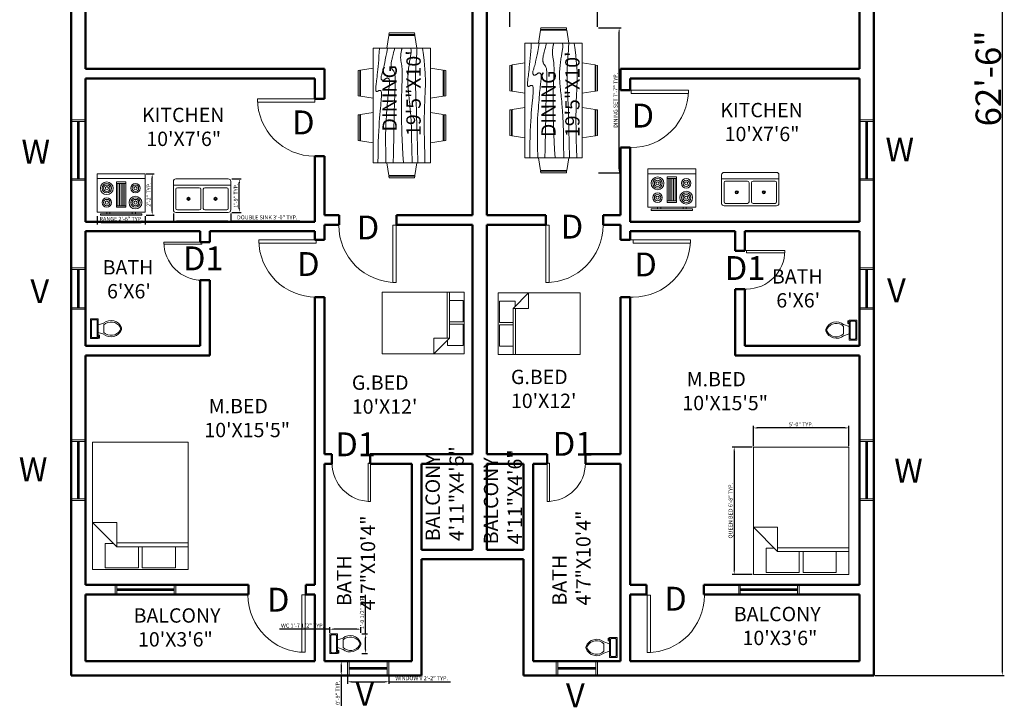
# Model space of a CAD drawing. Units: inches. Extents: x -7040 to -4088, y 6092 to 7645.
# Tile 10 of 11: x -4706 to -4088, y 6744 to 7176. Entities that reach past the tile are written whole.
import ezdxf

# ---------------------------------------------------------------- set-up
doc = ezdxf.new("R2010")
doc.units = ezdxf.units.IN
for name, color, linetype, lineweight in [('A-ANNO-DIMS', 2, 'Continuous', 18), ('A-ANNO-TEXT', 7, 'Continuous', 25), ('A-AREA-IDEN', 3, 'Continuous', 25), ('A-DOOR', 3, 'Continuous', 18), ('A-FLOR-FIXT', 9, 'Continuous', 13), ('A-FURN', 8, 'Continuous', 13), ('A-GLAZ', 4, 'Continuous', 18), ('A-WALL', 7, 'Continuous', 50)]:
    doc.layers.add(name, color=color, linetype=linetype, lineweight=lineweight)
doc.styles.get("Standard").update_dxf_attribs({"font": 'arial.ttf'})
doc.dimstyles.new('ISO-25', dxfattribs={"dimtxt": 2.5, "dimasz": 2.5, "dimexe": 1.25, "dimexo": 0.625, "dimtad": 1, "dimdec": 0, "dimlunit": 3, "dimtxsty": 'Standard', "dimcen": 2.5, "dimadec": 0, "dimazin": 0, "dimtfac": 1, "dimtdec": 0, "dimtmove": 0, "dimatfit": 3, "dimfxl": 1, "dimarcsym": 0})

# ---------------------------------------------------------------- blocks, each defined once
blk = doc.blocks.new('*U8')
for p, q in [((0, 0), (0, -100)), ((750, 0), (750, -100))]:
    blk.add_line(p, q)
blk.add_lwpolyline([(0, 0), (0, 750), (43.75, 750), (43.75, 0)], close=True)
blk.add_arc((0, 0), 750, 0, 90)
blk = doc.blocks.new('Bed - Queen')
for p, q in [((0, -80.00003), (0, 0)), ((0, 0), (59.99999, 0)), ((59.99999, 0), (59.99999, -80.00003)), ((7.99999, -1.2), (28.79998, -1.2)), ((7.99999, -14.4), (7.99999, -1.2)), ((28.79998, -1.2), (28.79998, -14.4)), ((31.19999, -1.2), (51.99999, -1.2)), ((31.19999, -14.4), (31.19999, -1.2)), ((51.99999, -1.2), (51.99999, -16.4)), ((0, -14.4), (44.8, -14.4)), ((44.8, -16.8), (0, -16.8)), ((59.99999, -29.6), (44.8, -14.4)), ((44.8, -14.4), (44.8, -29.6)), ((51.99999, -16.4), (46.79936, -16.4)), ((44.8, -29.6), (59.99999, -29.6)), ((59.99999, -80.00003), (0, -80.00003))]:
    blk.add_line(p, q)
blk = doc.blocks.new('Dining Set - 36 x 72 in.')
for p, q in [((-22.2343, 26.00059), (-23.4847, 17.99762)), ((-22.2304, 26), (-5.7608, 26)), ((-22, 27.5), (-22.1562, 26.50042)), ((-5.8416, 26.5), (-22.1534, 26.5)), ((-22, 27.5), (-6, 27.5)), ((-5.8437, 26.49966), (-6, 27.5)), ((-4.5152, 17.99762), (-5.7655, 25.99926)), ((5.7657, 26.00059), (4.5153, 17.99762)), ((5.7696, 26), (22.2392, 26)), ((6, 27.5), (5.8438, 26.50042)), ((22.1584, 26.5), (5.8466, 26.5)), ((6, 27.5), (22, 27.5)), ((22.1563, 26.49966), (22, 27.5)), ((23.4848, 17.99762), (22.2345, 25.99926)), ((36, 18), (-36, 18)), ((-36, 18), (-36, -18)), ((36, -18), (36, 18)), ((-45.5, 8), (-44.5004, 8.15617)), ((-45.5, 8), (-45.5, -8)), ((-44.5, -8.15843), (-44.5, 8.15338)), ((-44.0006, 8.23428), (-35.9976, 9.48474)), ((-44, 8.23041), (-44, -8.23915)), ((44.0006, 8.23428), (35.9976, 9.48474)), ((44, 8.23041), (44, -8.23915)), ((44.5, -8.15843), (44.5, 8.15338)), ((45.5, 8), (44.5005, 8.15617)), ((45.5, 8), (45.5, -8)), ((-44.4997, -8.15631), (-45.5, -8)), ((-35.9976, -9.48476), (-43.9993, -8.2345)), ((35.9976, -9.48476), (43.9993, -8.2345)), ((44.4997, -8.15631), (45.5, -8)), ((-36, -18), (36, -18)), ((-22.2343, -26.0006), (-23.4847, -17.99762)), ((-4.5152, -17.99762), (-5.7655, -25.99928)), ((5.7657, -26.0006), (4.5153, -17.99762)), ((23.4848, -17.99762), (22.2345, -25.99928)), ((-22.2304, -26), (-5.7608, -26)), ((-22, -27.5), (-22.1562, -26.50044)), ((-5.8416, -26.5), (-22.1534, -26.5)), ((-22, -27.5), (-6, -27.5)), ((-5.8437, -26.49967), (-6, -27.5)), ((5.7696, -26), (22.2392, -26)), ((6, -27.5), (5.8438, -26.50044)), ((22.1584, -26.5), (5.8466, -26.5)), ((6, -27.5), (22, -27.5)), ((22.1563, -26.49967), (22, -27.5))]:
    blk.add_line(p, q)
for points in [[(-36, 15), (-31.1772, 14.97754), (-26.8079, 14.91406), (-22.8538, 14.81543), (-19.276, 14.6875), (-16.0362, 14.53613), (-13.0957, 14.36718), (-10.4159, 14.18652), (-7.9583, 14), (-5.6904, 13.81315), (-3.6035, 13.63021), (-1.6954, 13.45508), (0.0365, 13.29166), (1.5945, 13.14388), (2.9811, 13.01562), (4.1988, 12.9108), (5.25, 12.83333), (6.1393, 12.78613), (6.8802, 12.76823), (7.4883, 12.77767), (7.9792, 12.8125), (8.3685, 12.87077), (8.6719, 12.95052), (8.9049, 13.0498), (9.0833, 13.16666), (9.2205, 13.29899), (9.3216, 13.44401), (9.3895, 13.59879), (9.4271, 13.76041), (9.4373, 13.92594), (9.4232, 14.09245), (9.3875, 14.257), (9.3333, 14.41666), (9.2638, 14.56917), (9.1836, 14.71484), (9.0975, 14.85465), (9.0104, 14.98958), (8.9272, 15.1206), (8.8529, 15.2487), (8.7922, 15.37483), (8.75, 15.5), (8.7305, 15.62467), (8.7344, 15.74739), (8.7617, 15.86621), (8.8125, 15.97916), (8.8867, 16.08431), (8.9844, 16.17968), (9.1055, 16.26334), (9.25, 16.33333), (9.4189, 16.38802), (9.6172, 16.42708), (9.8506, 16.45052), (10.125, 16.45833), (10.4463, 16.45052), (10.8203, 16.42708), (11.2529, 16.38802), (11.75, 16.33333), (12.3184, 16.26318), (12.9694, 16.17838), (13.7151, 16.07991), (14.5677, 15.96875), (15.5395, 15.84586), (16.6426, 15.71224), (17.8893, 15.56884), (19.2917, 15.41666), (20.859, 15.25667), (22.5879, 15.08984), (24.4721, 14.91715), (26.5052, 14.73958), (28.6809, 14.5581), (30.9929, 14.3737), (33.4347, 14.18733), (36, 14)], [(-36, 10), (-28.9766, 10.14274), (-23.1725, 10.20442), (-18.4241, 10.19775), (-14.5677, 10.13541), (-11.4399, 10.03011), (-8.877, 9.89453), (-6.7154, 9.74137), (-4.7917, 9.58333), (-2.9698, 9.43082), (-1.2246, 9.28515), (0.4415, 9.14534), (2.026, 9.01041), (3.5266, 8.87939), (4.9408, 8.7513), (6.266, 8.62516), (7.5, 8.5), (8.6411, 8.37549), (9.6914, 8.2539), (10.6538, 8.13818), (11.5312, 8.03125), (12.3267, 7.93603), (13.043, 7.85547), (13.6831, 7.79248), (14.25, 7.75), (14.7471, 7.7303), (15.1797, 7.73307), (15.5537, 7.75732), (15.875, 7.80208), (16.1494, 7.86637), (16.3828, 7.94922), (16.5811, 8.04964), (16.75, 8.16666), (16.8944, 8.29915), (17.0143, 8.44531), (17.1089, 8.60319), (17.1771, 8.77083), (17.218, 8.94629), (17.2305, 9.1276), (17.2137, 9.31282), (17.1667, 9.5), (17.0895, 9.6875), (16.987, 9.875), (16.8649, 10.0625), (16.7292, 10.25), (16.5856, 10.4375), (16.4401, 10.625), (16.2985, 10.8125), (16.1667, 11), (16.05, 11.18733), (15.9518, 11.3737), (15.8752, 11.5581), (15.8229, 11.73958), (15.798, 11.91715), (15.8034, 12.08984), (15.842, 12.25667), (15.9167, 12.41666), (16.0295, 12.56836), (16.1784, 12.70833), (16.3605, 12.83268), (16.5729, 12.9375), (16.8127, 13.01888), (17.0768, 13.07291), (17.3625, 13.0957), (17.6667, 13.08333), (17.9894, 13.03312), (18.3418, 12.94726), (18.7382, 12.82918), (19.1927, 12.68229), (19.7195, 12.51001), (20.3327, 12.31575), (21.0465, 12.10294), (21.875, 11.875), (22.8357, 11.63354), (23.959, 11.37304), (25.2786, 11.08618), (26.8282, 10.76562), (28.6414, 10.40405), (30.752, 9.99414), (33.1936, 9.52856), (36, 9)], [(-36, 5.5), (-30.7157, 5.3348), (-26.069, 5.20963), (-21.9946, 5.11767), (-18.4271, 5.05208), (-15.3009, 5.00602), (-12.5508, 4.97265), (-10.1112, 4.94515), (-7.9167, 4.91666), (-5.909, 4.88167), (-4.0586, 4.83984), (-2.3429, 4.79215), (-0.7396, 4.73958), (0.7739, 4.6831), (2.22, 4.6237), (3.6213, 4.56233), (5, 4.5), (6.373, 4.43782), (7.7344, 4.3776), (9.0723, 4.32129), (10.375, 4.27083), (11.6309, 4.22819), (12.8281, 4.19531), (13.9551, 4.17415), (15, 4.16666), (15.954, 4.17448), (16.819, 4.19791), (17.6001, 4.23698), (18.3021, 4.29166), (18.9299, 4.36198), (19.4883, 4.44791), (19.9823, 4.54948), (20.4167, 4.66666), (20.7969, 4.79899), (21.1302, 4.94401), (21.4245, 5.09879), (21.6875, 5.26041), (21.9271, 5.42594), (22.1511, 5.59245), (22.3672, 5.757), (22.5834, 5.91666), (22.8065, 6.06868), (23.0404, 6.21093), (23.2879, 6.34147), (23.5521, 6.45833), (23.8358, 6.55957), (24.142, 6.64323), (24.4735, 6.70735), (24.8334, 6.75), (25.2235, 6.76969), (25.642, 6.76692), (26.0858, 6.74267), (26.5521, 6.69791), (27.0379, 6.63362), (27.5404, 6.55078), (28.0565, 6.45036), (28.5834, 6.33333), (29.1242, 6.19987), (29.7071, 6.04687), (30.3661, 5.87044), (31.1354, 5.66666), (32.0493, 5.43164), (33.142, 5.16146), (34.4475, 4.85221), (36, 4.5)], [(-36, -1), (-30.7915, -0.6591), (-26.0195, -0.38216), (-21.6519, -0.16284), (-17.6563, 0.00521), (-14.0005, 0.12833), (-10.6523, 0.21289), (-7.5796, 0.26522), (-4.75, 0.29166), (-2.134, 0.29793), (0.2878, 0.28711), (2.5317, 0.26163), (4.6146, 0.22396), (6.5529, 0.17651), (8.3633, 0.12174), (10.0623, 0.06209), (11.6667, 0), (13.1899, -0.06201), (14.6341, -0.1211), (15.9982, -0.17432), (17.2813, -0.21875), (18.4823, -0.25147), (19.6003, -0.26953), (20.6343, -0.27002), (21.5834, -0.25), (22.4481, -0.20768), (23.2357, -0.14584), (23.9549, -0.06836), (24.6146, 0.02083), (25.2235, 0.11784), (25.7904, 0.21875), (26.3241, 0.31966), (26.8334, 0.41666), (27.3265, 0.50618), (27.8099, 0.58593), (28.2894, 0.65397), (28.7709, 0.70833), (29.2601, 0.74707), (29.763, 0.76823), (30.2855, 0.76985), (30.8334, 0.75), (31.4088, 0.70784), (31.9994, 0.64713), (32.589, 0.57275), (33.1615, 0.48958), (33.7008, 0.4025), (34.1908, 0.3164), (34.6153, 0.23616), (34.9584, 0.16666), (35.2099, 0.11165), (35.3848, 0.07031), (35.504, 0.04069), (35.5886, 0.02083), (35.6594, 0.00879), (35.7377, 0.0026), (35.8442, 0.00032), (36, 0)], [(-36, -6.5), (-27.1843, -6.31267), (-20.084, -6.1263), (-14.469, -5.9419), (-10.1094, -5.76042), (-6.7752, -5.58285), (-4.2363, -5.41016), (-2.2629, -5.24333), (-0.625, -5.08334), (0.8708, -4.93099), (2.2715, -4.78646), (3.5872, -4.64974), (4.8281, -4.52084), (6.0046, -4.39974), (7.127, -4.28646), (8.2053, -4.18099), (9.25, -4.08334), (10.2705, -3.99382), (11.2734, -3.91407), (12.2647, -3.84603), (13.25, -3.79167), (14.2354, -3.75293), (15.2266, -3.73177), (16.2295, -3.73015), (17.25, -3.75), (18.2912, -3.79248), (19.3451, -3.85547), (20.4009, -3.93604), (21.4479, -4.03125), (22.4754, -4.13819), (23.4727, -4.25391), (24.4289, -4.37549), (25.3334, -4.5), (26.1785, -4.62492), (26.9694, -4.74935), (27.7145, -4.87281), (28.4219, -4.99479), (29.1, -5.11483), (29.7572, -5.23242), (30.4016, -5.34709), (31.0417, -5.45834), (31.6837, -5.56437), (32.3262, -5.65821), (32.9658, -5.73153), (33.599, -5.77604), (34.2224, -5.78345), (34.8327, -5.74545), (35.4264, -5.65373), (36, -5.5)], [(-36, -10), (-26.4022, -9.81299), (-18.4675, -9.62891), (-11.9839, -9.45069), (-6.7396, -9.28125), (-2.5226, -9.12354), (0.8789, -8.98047), (3.6769, -8.85498), (6.0833, -8.75), (8.2767, -8.66765), (10.3021, -8.60677), (12.1712, -8.56543), (13.8958, -8.54167), (15.4876, -8.53353), (16.9583, -8.53907), (18.3197, -8.55632), (19.5834, -8.58334), (20.7616, -8.61841), (21.8685, -8.66081), (22.9188, -8.71004), (23.9271, -8.76563), (24.9081, -8.82707), (25.8763, -8.89388), (26.8465, -8.96558), (27.8334, -9.04167), (28.8474, -9.12118), (29.8828, -9.20117), (30.93, -9.27824), (31.9792, -9.34896), (33.0205, -9.40991), (34.0443, -9.45768), (35.0407, -9.48885), (36, -9.5)], [(-36, -14.5), (-30.0881, -14.33513), (-25.0332, -14.21224), (-20.7312, -14.12647), (-17.0781, -14.07292), (-13.97, -14.04671), (-11.3027, -14.04297), (-8.9724, -14.05681), (-6.875, -14.08334), (-4.9224, -14.11833), (-3.0905, -14.16016), (-1.3709, -14.20785), (0.2448, -14.26042), (1.7647, -14.3169), (3.1973, -14.3763), (4.5507, -14.43767), (5.8333, -14.5), (7.0554, -14.5621), (8.235, -14.62175), (9.3922, -14.67652), (10.5469, -14.72396), (11.7192, -14.76164), (12.929, -14.78711), (14.1965, -14.79794), (15.5417, -14.79167), (16.9933, -14.76424), (18.6152, -14.70508), (20.4804, -14.60197), (22.6615, -14.44271), (25.2312, -14.21509), (28.2624, -13.9069), (31.8277, -13.50594), (36, -13)]]:
    blk.add_lwpolyline(points)
blk = doc.blocks.new('Toilet - top')
for p, q in [((-10, -8.5), (-8, -8.5)), ((-10, -9.5), (-10, -8.5)), ((-7, -9.5), (-10, -9.5)), ((-8, -8.5), (-8, -8)), ((-7, -8), (-7, -9.5)), ((-4, -8), (-6, -14)), ((4, -8), (6, -14)), ((9.5, -6), (9.5, -2)), ((4, -14), (-4, -14))]:
    blk.add_line(p, q)
blk.add_lwpolyline([(10.5, -8), (10.5, 0), (-10.5, 0), (-10.5, -8)], close=True)
for points in [[(-9.5, -2), (-9.5, -6)], [(8.5, -1), (-8.5, -1)], [(-8.5, -7), (8.5, -7)]]:
    blk.add_lwpolyline(points)
for centre, radius, start, end in [((-8.6, -1.9), 0.884, 81.8699, 188.1301), ((-8.6, -6.1), 0.884, 171.8699, 278.1301), ((8.6, -1.9), 0.884, 351.8699, 98.1301), ((8.6, -6.1), 0.884, 261.8699, 8.1301), ((3.5, -21.6), 12.2, 141.4691, 247.9714), ((4.2, -21.8), 11.3, 136.3677, 238.9468), ((-3.5, -21.6), 12.2, 292.0284, 38.5307), ((-4.2, -21.8), 11.3, 301.053, 43.6321), ((0, -27.9), 4, 245.7318, 294.2682), ((0, -29), 4, 254.8605, 285.1395)]:
    blk.add_arc(centre, radius, start, end)
blk = doc.blocks.new('Range-Oven - 30 in top')
for p, q in [((0, -3), (30, -3)), ((12, -6), (18, -6)), ((13, -20), (13, -6)), ((14, -6), (14, -20)), ((15, -20), (15, -6)), ((16, -6), (16, -20)), ((17, -20), (17, -6)), ((6, -24), (6, -25)), ((8, -25), (8, -24)), ((18, -20), (12, -20)), ((22, -25), (22, -24)), ((24, -24), (24, -25))]:
    blk.add_line(p, q)
for points in [[(0, -24), (0, 0), (30, 0), (30, -24)], [(12, -21), (12, -5), (18, -5), (18, -21)], [(2, -26), (2, -25), (28, -25), (28, -26)]]:
    blk.add_lwpolyline(points, close=True)
for centre, radius in [((6, -9), 4), ((6, -9), 3), ((24, -9), 3), ((6, -9), 2), ((6, -9), 1), ((24, -9), 2), ((24, -9), 1), ((6, -18), 3), ((6, -18), 2), ((6, -18), 1), ((24, -18), 4), ((24, -18), 3), ((24, -18), 2), ((24, -18), 1)]:
    blk.add_circle(centre, radius)
blk = doc.blocks.new('Sink-double - 36 in top')
for p, q in [((-18, -4), (18, -4)), ((-0.75, -18.5), (-0.75, -6.5)), ((0.75, -6.5), (0.75, -18.5))]:
    blk.add_line(p, q)
for points in [[(-16.5, 0), (16.5, 0)], [(-18, -19.5), (-18, -1.5)], [(-15.5, -5.5), (-1.75, -5.5)], [(1.75, -5.5), (15.5, -5.5)], [(18, -1.5), (18, -19.5)], [(-16.5, -18.5), (-16.5, -6.5)], [(16.5, -6.5), (16.5, -18.5)], [(16.5, -21), (-16.5, -21)], [(-1.75, -19.5), (-15.5, -19.5)], [(15.5, -19.5), (1.75, -19.5)]]:
    blk.add_lwpolyline(points)
for centre, radius in [((-8.5, -12.5), 1), ((-8.5, -12.5), 0.5), ((8.5, -12.5), 1), ((8.5, -12.5), 0.5)]:
    blk.add_circle(centre, radius)
for centre, radius, start, end in [((-16.5, -1.5), 1.5, 90, 180), ((16.5, -1.5), 1.5, 0, 90), ((-15.5, -6.5), 1, 90, 180), ((-1.75, -6.5), 1, 0, 90), ((1.75, -6.5), 1, 90, 180), ((15.5, -6.5), 1, 0, 90), ((-15.5, -18.5), 1, 180, 270), ((-1.75, -18.5), 1, 270, 0), ((1.75, -18.5), 1, 180, 270), ((15.5, -18.5), 1, 270, 0), ((-16.5, -19.5), 1.5, 180, 270), ((16.5, -19.5), 1.5, 270, 0)]:
    blk.add_arc(centre, radius, start, end)
blk = doc.blocks.new('*D109')
at = {"layer": 'A-ANNO-DIMS', "color": 0, "lineweight": -2, "transparency": 16777216}
for p, q in [((-4169.15, 7513.76), (-4087.83, 7513.76)), ((-4089.08, 7511.26), (-4089.08, 6766.26)), ((-4169.15, 6763.76), (-4087.83, 6763.76))]:
    blk.add_line(p, q, dxfattribs=at)
at = {"layer": 'A-ANNO-DIMS', "color": 0, "transparency": 16777216}
for points in [[(-4089.49, 7511.26), (-4088.66, 7511.26), (-4089.08, 7513.76)], [(-4089.49, 6766.26), (-4088.66, 6766.26), (-4089.08, 6763.76)]]:
    blk.add_solid(points, dxfattribs=at)
at = {"layer": 'Defpoints', "color": 0, "transparency": 16777216}
for p in [(-4169.77, 7513.76), (-4169.77, 6763.76), (-4089.08, 6763.76)]:
    blk.add_point(p, dxfattribs=at)
at = {"layer": 'A-ANNO-DIMS', "color": 0, "transparency": 16777216, "insert": (-4097.87, 7138.76), "char_height": 2.5, "attachment_point": 5, "rotation": 90}
blk.add_mtext('{\\H6.4x;62\'-6"}', dxfattribs=at)
blk = doc.blocks.new('WIN-36')
for p, q in [((0, 6), (0, 0)), ((1, 6), (1, 0)), ((1, 3.5), (37, 3.5)), ((1, 3), (37, 3)), ((1, 2.5), (37, 2.5)), ((37, 6), (37, 0)), ((38, 6), (38, 0))]:
    blk.add_line(p, q)
blk = doc.blocks.new('WIN-36-B')
for p, q in [((0, 38), (9, 38)), ((0, 37), (9, 37)), ((4, 1), (4, 37)), ((4.5, 1), (4.5, 37)), ((5, 1), (5, 37)), ((0, 1), (9, 1)), ((0, 0), (9, 0))]:
    blk.add_line(p, q)
blk = doc.blocks.new('WIN-24-B')
for p, q in [((0, 26), (9, 26)), ((0, 25), (9, 25)), ((4, 1), (4, 25)), ((4.5, 1), (4.5, 25)), ((5, 1), (5, 25)), ((0, 1), (9, 1)), ((0, 0), (9, 0))]:
    blk.add_line(p, q)
blk = doc.blocks.new('*D120')
at = {"layer": 'A-ANNO-DIMS', "color": 0, "lineweight": -2, "transparency": 16777216}
for p, q in [((-4500.27, 6763.13), (-4500.27, 6758.61)), ((-4497.77, 6759.86), (-4476.77, 6759.86)), ((-4474.27, 6763.13), (-4474.27, 6758.61)), ((-4474.27, 6759.86), (-4435.59, 6759.86))]:
    blk.add_line(p, q, dxfattribs=at)
at = {"layer": 'A-ANNO-DIMS', "color": 0, "transparency": 16777216}
for points in [[(-4497.77, 6760.28), (-4497.77, 6759.44), (-4500.27, 6759.86)], [(-4476.77, 6760.28), (-4476.77, 6759.44), (-4474.27, 6759.86)]]:
    blk.add_solid(points, dxfattribs=at)
at = {"layer": 'Defpoints', "color": 0, "transparency": 16777216}
for p in [(-4500.27, 6763.76), (-4474.27, 6763.76), (-4474.27, 6759.86)]:
    blk.add_point(p, dxfattribs=at)
at = {"layer": 'A-ANNO-DIMS', "color": 0, "transparency": 16777216, "insert": (-4453.68, 6761.78), "char_height": 2.5, "attachment_point": 5}
blk.add_mtext('WINDOW V 2\'-2" TYP.', dxfattribs=at)
blk = doc.blocks.new('*D121')
at = {"layer": 'A-ANNO-DIMS', "color": 0, "lineweight": -2, "transparency": 16777216}
for p, q in [((-4500.9, 6772.76), (-4505.42, 6772.76)), ((-4504.17, 6770.26), (-4504.17, 6766.26)), ((-4500.9, 6763.76), (-4505.42, 6763.76)), ((-4504.17, 6763.76), (-4504.17, 6744.77))]:
    blk.add_line(p, q, dxfattribs=at)
at = {"layer": 'A-ANNO-DIMS', "color": 0, "transparency": 16777216}
for points in [[(-4504.59, 6770.26), (-4503.76, 6770.26), (-4504.17, 6772.76)], [(-4504.59, 6766.26), (-4503.76, 6766.26), (-4504.17, 6763.76)]]:
    blk.add_solid(points, dxfattribs=at)
at = {"layer": 'Defpoints', "color": 0, "transparency": 16777216}
for p in [(-4500.27, 6772.76), (-4504.17, 6763.76), (-4500.27, 6763.76)]:
    blk.add_point(p, dxfattribs=at)
at = {"layer": 'A-ANNO-DIMS', "color": 0, "transparency": 16777216, "insert": (-4506.07, 6753.01), "char_height": 2.5, "attachment_point": 5, "rotation": 90}
blk.add_mtext('0\'-9" TYP.', dxfattribs=at)
blk = doc.blocks.new('*D126')
at = {"layer": 'A-ANNO-DIMS', "color": 0, "lineweight": -2, "transparency": 16777216}
for p, q in [((-4246.05, 6907.26), (-4258.67, 6907.26)), ((-4257.42, 6904.76), (-4257.42, 6829.76)), ((-4246.05, 6827.26), (-4258.67, 6827.26))]:
    blk.add_line(p, q, dxfattribs=at)
at = {"layer": 'A-ANNO-DIMS', "color": 0, "transparency": 16777216}
for points in [[(-4257.84, 6904.76), (-4257.01, 6904.76), (-4257.42, 6907.26)], [(-4257.84, 6829.76), (-4257.01, 6829.76), (-4257.42, 6827.26)]]:
    blk.add_solid(points, dxfattribs=at)
at = {"layer": 'Defpoints', "color": 0, "transparency": 16777216}
for p in [(-4245.42, 6907.26), (-4257.42, 6827.26), (-4245.42, 6827.26)]:
    blk.add_point(p, dxfattribs=at)
at = {"layer": 'A-ANNO-DIMS', "color": 0, "transparency": 16777216, "insert": (-4259.42, 6867.26), "char_height": 2.5, "attachment_point": 5, "rotation": 90}
blk.add_mtext('QUEEN BED 6\'-8" TYP.', dxfattribs=at)
blk = doc.blocks.new('*D127')
at = {"layer": 'A-ANNO-DIMS', "color": 0, "lineweight": -2, "transparency": 16777216}
for p, q in [((-4245.42, 6907.88), (-4245.42, 6920.51)), ((-4187.92, 6919.26), (-4242.92, 6919.26)), ((-4185.42, 6907.88), (-4185.42, 6920.51))]:
    blk.add_line(p, q, dxfattribs=at)
at = {"layer": 'A-ANNO-DIMS', "color": 0, "transparency": 16777216}
for points in [[(-4242.92, 6919.67), (-4242.92, 6918.84), (-4245.42, 6919.26)], [(-4187.92, 6919.67), (-4187.92, 6918.84), (-4185.42, 6919.26)]]:
    blk.add_solid(points, dxfattribs=at)
at = {"layer": 'Defpoints', "color": 0, "transparency": 16777216}
for p in [(-4245.42, 6919.26), (-4245.42, 6907.26), (-4185.42, 6907.26)]:
    blk.add_point(p, dxfattribs=at)
at = {"layer": 'A-ANNO-DIMS', "color": 0, "transparency": 16777216, "insert": (-4215.42, 6921.16), "char_height": 2.5, "attachment_point": 5}
blk.add_mtext('5\'-0" TYP.', dxfattribs=at)
blk = doc.blocks.new('*D132')
at = {"layer": 'A-ANNO-DIMS', "color": 0, "lineweight": -2, "transparency": 16777216}
for p, q in [((-4511.36, 6792.89), (-4543.06, 6792.89)), ((-4511.36, 6790.58), (-4511.36, 6794.14)), ((-4494.3, 6792.89), (-4508.86, 6792.89)), ((-4491.8, 6790.58), (-4491.8, 6794.14))]:
    blk.add_line(p, q, dxfattribs=at)
at = {"layer": 'A-ANNO-DIMS', "color": 0, "transparency": 16777216}
for points in [[(-4508.86, 6793.31), (-4508.86, 6792.47), (-4511.36, 6792.89)], [(-4494.3, 6793.31), (-4494.3, 6792.47), (-4491.8, 6792.89)]]:
    blk.add_solid(points, dxfattribs=at)
at = {"layer": 'Defpoints', "color": 0, "transparency": 16777216}
for p in [(-4511.36, 6792.89), (-4511.36, 6789.96), (-4491.8, 6789.96)]:
    blk.add_point(p, dxfattribs=at)
at = {"layer": 'A-ANNO-DIMS', "color": 0, "transparency": 16777216, "insert": (-4528.46, 6794.81), "char_height": 2.5, "attachment_point": 5}
blk.add_mtext('WC 1\'-7 1/2" TYP.', dxfattribs=at)
blk = doc.blocks.new('*D133')
at = {"layer": 'A-ANNO-DIMS', "color": 0, "lineweight": -2, "transparency": 16777216}
for p, q in [((-4488.87, 6789.96), (-4488.87, 6814.54)), ((-4491.18, 6789.96), (-4487.62, 6789.96)), ((-4488.87, 6780.03), (-4488.87, 6787.46)), ((-4491.18, 6777.53), (-4487.62, 6777.53))]:
    blk.add_line(p, q, dxfattribs=at)
at = {"layer": 'A-ANNO-DIMS', "color": 0, "transparency": 16777216}
for points in [[(-4489.28, 6787.46), (-4488.45, 6787.46), (-4488.87, 6789.96)], [(-4489.28, 6780.03), (-4488.45, 6780.03), (-4488.87, 6777.53)]]:
    blk.add_solid(points, dxfattribs=at)
at = {"layer": 'Defpoints', "color": 0, "transparency": 16777216}
for p in [(-4491.8, 6789.96), (-4488.87, 6789.96), (-4491.8, 6777.53)]:
    blk.add_point(p, dxfattribs=at)
at = {"layer": 'A-ANNO-DIMS', "color": 0, "transparency": 16777216, "insert": (-4490.79, 6803.5), "char_height": 2.5, "attachment_point": 5, "rotation": 90}
blk.add_mtext('1\'-0 1/2" TYP.', dxfattribs=at)
blk = doc.blocks.new('*D146')
at = {"layer": 'A-ANNO-DIMS', "color": 0, "lineweight": -2, "transparency": 16777216}
for p, q in [((-4342.71, 7170.43), (-4328.44, 7170.43)), ((-4329.69, 7081.93), (-4329.69, 7167.93)), ((-4342.71, 7079.43), (-4328.44, 7079.43))]:
    blk.add_line(p, q, dxfattribs=at)
at = {"layer": 'A-ANNO-DIMS', "color": 0, "transparency": 16777216}
for points in [[(-4330.1, 7167.93), (-4329.27, 7167.93), (-4329.69, 7170.43)], [(-4330.1, 7081.93), (-4329.27, 7081.93), (-4329.69, 7079.43)]]:
    blk.add_solid(points, dxfattribs=at)
at = {"layer": 'Defpoints', "color": 0, "transparency": 16777216}
for p in [(-4343.34, 7170.43), (-4329.69, 7170.43), (-4343.34, 7079.43)]:
    blk.add_point(p, dxfattribs=at)
at = {"layer": 'A-ANNO-DIMS', "color": 0, "transparency": 16777216, "insert": (-4331.6, 7124.93), "char_height": 2.5, "attachment_point": 5, "rotation": 90}
blk.add_mtext('DINING SET 7\'-7" TYP.', dxfattribs=at)
blk = doc.blocks.new('*D147')
at = {"layer": 'A-ANNO-DIMS', "color": 0, "lineweight": -2, "transparency": 16777216}
for p, q in [((-4398.34, 7171.05), (-4398.34, 7185.33)), ((-4343.34, 7171.05), (-4343.34, 7185.33)), ((-4345.84, 7184.08), (-4395.84, 7184.08))]:
    blk.add_line(p, q, dxfattribs=at)
at = {"layer": 'A-ANNO-DIMS', "color": 0, "transparency": 16777216}
for points in [[(-4395.84, 7184.49), (-4395.84, 7183.66), (-4398.34, 7184.08)], [(-4345.84, 7184.49), (-4345.84, 7183.66), (-4343.34, 7184.08)]]:
    blk.add_solid(points, dxfattribs=at)
at = {"layer": 'Defpoints', "color": 0, "transparency": 16777216}
for p in [(-4398.34, 7184.08), (-4398.34, 7170.43), (-4343.34, 7170.43)]:
    blk.add_point(p, dxfattribs=at)
at = {"layer": 'A-ANNO-DIMS', "color": 0, "transparency": 16777216, "insert": (-4370.84, 7185.95), "char_height": 2.5, "attachment_point": 5}
blk.add_mtext('4\'-7" TYP.', dxfattribs=at)
blk = doc.blocks.new('*D152')
at = {"layer": 'A-ANNO-DIMS', "color": 0, "lineweight": -2, "transparency": 16777216}
for p, q in [((-4657.4, 7052.16), (-4657.4, 7047.03)), ((-4627.4, 7052.16), (-4627.4, 7047.03)), ((-4654.9, 7048.28), (-4629.9, 7048.28))]:
    blk.add_line(p, q, dxfattribs=at)
at = {"layer": 'A-ANNO-DIMS', "color": 0, "transparency": 16777216}
for points in [[(-4654.9, 7048.7), (-4654.9, 7047.87), (-4657.4, 7048.28)], [(-4629.9, 7048.7), (-4629.9, 7047.87), (-4627.4, 7048.28)]]:
    blk.add_solid(points, dxfattribs=at)
at = {"layer": 'Defpoints', "color": 0, "transparency": 16777216}
for p in [(-4657.4, 7052.78), (-4627.4, 7052.78), (-4627.4, 7048.28)]:
    blk.add_point(p, dxfattribs=at)
at = {"layer": 'A-ANNO-DIMS', "color": 0, "transparency": 16777216, "insert": (-4642.4, 7050.2), "char_height": 2.5, "attachment_point": 5}
blk.add_mtext('RANGE 2\'-6" TYP.', dxfattribs=at)
blk = doc.blocks.new('*D153')
at = {"layer": 'A-ANNO-DIMS', "color": 0, "lineweight": -2, "transparency": 16777216}
for p, q in [((-4626.77, 7078.78), (-4621.65, 7078.78)), ((-4622.9, 7055.28), (-4622.9, 7076.28)), ((-4626.77, 7052.78), (-4621.65, 7052.78))]:
    blk.add_line(p, q, dxfattribs=at)
at = {"layer": 'A-ANNO-DIMS', "color": 0, "transparency": 16777216}
for points in [[(-4623.31, 7076.28), (-4622.48, 7076.28), (-4622.9, 7078.78)], [(-4623.31, 7055.28), (-4622.48, 7055.28), (-4622.9, 7052.78)]]:
    blk.add_solid(points, dxfattribs=at)
at = {"layer": 'Defpoints', "color": 0, "transparency": 16777216}
for p in [(-4627.4, 7078.78), (-4622.9, 7078.78), (-4627.4, 7052.78)]:
    blk.add_point(p, dxfattribs=at)
at = {"layer": 'A-ANNO-DIMS', "color": 0, "transparency": 16777216, "insert": (-4624.78, 7065.78), "char_height": 2.5, "attachment_point": 5, "rotation": 90}
blk.add_mtext('2\'-2" TYP.', dxfattribs=at)
blk = doc.blocks.new('*D158')
at = {"layer": 'A-ANNO-DIMS', "color": 0, "lineweight": -2, "transparency": 16777216}
for p, q in [((-4609.59, 7053.98), (-4609.59, 7047.96)), ((-4607.09, 7049.21), (-4576.09, 7049.21)), ((-4573.59, 7053.98), (-4573.59, 7047.96)), ((-4573.59, 7049.21), (-4530.27, 7049.21))]:
    blk.add_line(p, q, dxfattribs=at)
at = {"layer": 'A-ANNO-DIMS', "color": 0, "transparency": 16777216}
for points in [[(-4607.09, 7049.62), (-4607.09, 7048.79), (-4609.59, 7049.21)], [(-4576.09, 7049.62), (-4576.09, 7048.79), (-4573.59, 7049.21)]]:
    blk.add_solid(points, dxfattribs=at)
at = {"layer": 'Defpoints', "color": 0, "transparency": 16777216}
for p in [(-4609.59, 7054.61), (-4573.59, 7054.61), (-4573.59, 7049.21)]:
    blk.add_point(p, dxfattribs=at)
at = {"layer": 'A-ANNO-DIMS', "color": 0, "transparency": 16777216, "insert": (-4550.68, 7051.13), "char_height": 2.5, "attachment_point": 5}
blk.add_mtext('DOUBLE SINK 3\'-0" TYP.', dxfattribs=at)
blk = doc.blocks.new('*D159')
at = {"layer": 'A-ANNO-DIMS', "color": 0, "lineweight": -2, "transparency": 16777216}
for p, q in [((-4572.96, 7075.61), (-4566.94, 7075.61)), ((-4568.19, 7057.11), (-4568.19, 7073.11)), ((-4572.96, 7054.61), (-4566.94, 7054.61))]:
    blk.add_line(p, q, dxfattribs=at)
at = {"layer": 'A-ANNO-DIMS', "color": 0, "transparency": 16777216}
for points in [[(-4568.6, 7073.11), (-4567.77, 7073.11), (-4568.19, 7075.61)], [(-4568.6, 7057.11), (-4567.77, 7057.11), (-4568.19, 7054.61)]]:
    blk.add_solid(points, dxfattribs=at)
at = {"layer": 'Defpoints', "color": 0, "transparency": 16777216}
for p in [(-4573.59, 7075.61), (-4568.19, 7075.61), (-4573.59, 7054.61)]:
    blk.add_point(p, dxfattribs=at)
at = {"layer": 'A-ANNO-DIMS', "color": 0, "transparency": 16777216, "insert": (-4570.09, 7065.11), "char_height": 2.5, "attachment_point": 5, "rotation": 90}
blk.add_mtext('1\'-9" TYP.', dxfattribs=at)

msp = doc.modelspace()

# ---------------------------------------------------------------- linework, layer by layer
at = {"layer": 'A-WALL'}
for p, q in [((-4673.77, 6763.76), (-4673.77, 7513.76)), ((-4169.77, 7513.76), (-4169.77, 6763.76)), ((-4664.77, 7144.76), (-4664.77, 7294.76)), ((-4178.77, 7294.76), (-4178.77, 7144.76)), ((-4421.77, 7246.46), (-4421.77, 7052.76)), ((-4412.77, 7246.46), (-4412.77, 7052.76)), ((-4664.77, 7144.76), (-4514.77, 7144.76)), ((-4514.77, 7125.86), (-4514.77, 7144.76)), ((-4328.77, 7144.76), (-4178.77, 7144.76)), ((-4328.77, 7144.76), (-4328.77, 7131.29)), ((-4664.77, 7138.76), (-4520.77, 7138.76)), ((-4664.77, 7048.76), (-4664.77, 7138.76)), ((-4520.77, 7125.86), (-4520.77, 7138.76)), ((-4322.77, 7138.76), (-4178.77, 7138.76)), ((-4322.77, 7138.76), (-4322.77, 7131.29)), ((-4178.77, 7138.76), (-4178.77, 7048.76)), ((-4328.77, 7131.29), (-4322.77, 7131.29)), ((-4520.77, 7125.86), (-4514.77, 7125.86)), ((-4328.77, 7095.29), (-4322.77, 7095.29)), ((-4328.77, 7095.29), (-4328.77, 7052.76)), ((-4322.77, 7095.29), (-4322.77, 7048.76)), ((-4520.77, 7048.76), (-4520.77, 7089.86)), ((-4520.77, 7089.86), (-4514.77, 7089.86)), ((-4514.77, 7052.76), (-4514.77, 7089.86)), ((-4664.77, 7048.76), (-4520.77, 7048.76)), ((-4505.48, 7052.76), (-4514.77, 7052.76)), ((-4505.48, 7052.76), (-4505.48, 7046.76)), ((-4421.77, 7052.76), (-4469.48, 7052.76)), ((-4469.48, 7052.76), (-4469.48, 7046.76)), ((-4375.62, 7052.76), (-4412.77, 7052.76)), ((-4375.62, 7052.76), (-4375.62, 7046.76)), ((-4328.77, 7052.76), (-4339.62, 7052.76)), ((-4339.62, 7052.76), (-4339.62, 7046.76)), ((-4322.77, 7048.76), (-4178.77, 7048.76)), ((-4664.77, 7042.76), (-4592.77, 7042.76)), ((-4664.77, 6970.76), (-4664.77, 7042.76)), ((-4592.77, 7035.95), (-4592.77, 7042.76)), ((-4586.77, 7042.76), (-4520.77, 7042.76)), ((-4586.77, 7035.95), (-4586.77, 7042.76)), ((-4520.77, 7037.38), (-4520.77, 7042.76)), ((-4505.48, 7046.76), (-4514.77, 7046.76)), ((-4514.77, 7037.38), (-4514.77, 7046.76)), ((-4421.77, 7046.76), (-4469.48, 7046.76)), ((-4421.77, 7046.76), (-4421.77, 6902.76)), ((-4412.77, 7046.76), (-4412.77, 6902.76)), ((-4375.62, 7046.76), (-4412.77, 7046.76)), ((-4328.77, 7046.76), (-4339.62, 7046.76)), ((-4328.77, 7046.76), (-4328.77, 7037.42)), ((-4322.77, 7042.76), (-4256.77, 7042.76)), ((-4322.77, 7042.76), (-4322.77, 7037.42)), ((-4256.77, 7042.76), (-4256.77, 7030.47)), ((-4250.77, 7042.76), (-4250.77, 7030.47)), ((-4250.77, 7042.76), (-4178.77, 7042.76)), ((-4178.77, 7042.76), (-4178.77, 6970.76)), ((-4520.77, 7037.38), (-4514.77, 7037.38)), ((-4328.77, 7037.42), (-4322.77, 7037.42)), ((-4592.77, 7035.95), (-4586.77, 7035.95)), ((-4256.77, 7030.47), (-4250.77, 7030.47)), ((-4592.77, 6970.76), (-4592.77, 7011.95)), ((-4592.77, 7011.95), (-4586.77, 7011.95)), ((-4586.77, 6964.76), (-4586.77, 7011.95)), ((-4256.77, 7006.47), (-4250.77, 7006.47)), ((-4256.77, 7006.47), (-4256.77, 6964.76)), ((-4250.77, 7006.47), (-4250.77, 6970.76)), ((-4520.77, 6820.76), (-4520.77, 7001.38)), ((-4520.77, 7001.38), (-4514.77, 7001.38)), ((-4514.77, 6902.76), (-4514.77, 7001.38)), ((-4328.77, 7001.42), (-4322.77, 7001.42)), ((-4328.77, 7001.42), (-4328.77, 6902.76)), ((-4322.77, 7001.42), (-4322.77, 6820.76)), ((-4664.77, 6970.76), (-4592.77, 6970.76)), ((-4250.77, 6970.76), (-4178.77, 6970.76)), ((-4664.77, 6964.76), (-4586.77, 6964.76)), ((-4664.77, 6820.76), (-4664.77, 6964.76)), ((-4256.77, 6964.76), (-4178.77, 6964.76)), ((-4178.77, 6964.76), (-4178.77, 6820.76)), ((-4510, 6902.76), (-4514.77, 6902.76)), ((-4510, 6902.76), (-4514.77, 6902.76)), ((-4510, 6902.76), (-4510, 6896.76)), ((-4453.77, 6902.76), (-4486, 6902.76)), ((-4421.77, 6902.76), (-4486, 6902.76)), ((-4486, 6902.76), (-4486, 6896.76)), ((-4383.77, 6902.76), (-4412.77, 6902.76)), ((-4374.86, 6902.76), (-4383.77, 6902.76)), ((-4374.86, 6902.76), (-4374.86, 6896.76)), ((-4328.77, 6902.76), (-4350.86, 6902.76)), ((-4350.86, 6902.76), (-4350.86, 6896.76)), ((-4514.77, 6772.76), (-4514.77, 6896.76)), ((-4510, 6896.76), (-4514.77, 6896.76)), ((-4510, 6896.76), (-4514.77, 6896.76)), ((-4459.77, 6896.76), (-4486, 6896.76)), ((-4459.77, 6896.76), (-4486, 6896.76)), ((-4459.77, 6772.76), (-4459.77, 6896.76)), ((-4421.77, 6896.76), (-4453.77, 6896.76)), ((-4453.77, 6842.76), (-4453.77, 6896.76)), ((-4421.77, 6896.76), (-4421.77, 6842.76)), ((-4389.77, 6896.76), (-4412.77, 6896.76)), ((-4412.77, 6896.76), (-4412.77, 6842.76)), ((-4389.77, 6896.76), (-4389.77, 6842.76)), ((-4383.77, 6896.76), (-4383.77, 6772.76)), ((-4374.86, 6896.76), (-4383.77, 6896.76)), ((-4328.77, 6896.76), (-4350.86, 6896.76)), ((-4328.77, 6896.76), (-4328.77, 6772.76)), ((-4421.77, 6842.76), (-4453.77, 6842.76)), ((-4389.77, 6842.76), (-4412.77, 6842.76)), ((-4453.77, 6763.76), (-4453.77, 6836.76)), ((-4389.77, 6836.76), (-4453.77, 6836.76)), ((-4389.77, 6836.76), (-4389.77, 6763.76)), ((-4562.5, 6820.76), (-4664.77, 6820.76)), ((-4562.5, 6820.76), (-4664.77, 6820.76)), ((-4562.5, 6820.76), (-4562.5, 6814.76)), ((-4520.77, 6820.76), (-4526.5, 6820.76)), ((-4520.77, 6820.76), (-4526.5, 6820.76)), ((-4526.5, 6820.76), (-4526.5, 6814.76)), ((-4312.55, 6820.76), (-4322.77, 6820.76)), ((-4312.55, 6820.76), (-4312.55, 6814.76)), ((-4178.77, 6820.76), (-4276.55, 6820.76)), ((-4276.55, 6820.76), (-4276.55, 6814.76)), ((-4664.77, 6772.76), (-4664.77, 6814.76)), ((-4562.5, 6814.76), (-4664.77, 6814.76)), ((-4562.5, 6814.76), (-4664.77, 6814.76)), ((-4520.77, 6814.76), (-4526.5, 6814.76)), ((-4520.77, 6814.76), (-4526.5, 6814.76)), ((-4520.77, 6772.76), (-4520.77, 6814.76)), ((-4322.77, 6814.76), (-4322.77, 6772.76)), ((-4312.55, 6814.76), (-4322.77, 6814.76)), ((-4178.77, 6814.76), (-4276.55, 6814.76)), ((-4178.77, 6814.76), (-4178.77, 6772.76)), ((-4520.77, 6772.76), (-4664.77, 6772.76)), ((-4459.77, 6772.76), (-4514.77, 6772.76)), ((-4328.77, 6772.76), (-4383.77, 6772.76)), ((-4178.77, 6772.76), (-4322.77, 6772.76)), ((-4453.77, 6763.76), (-4673.77, 6763.76)), ((-4169.77, 6763.76), (-4389.77, 6763.76))]:
    msp.add_line(p, q, dxfattribs=at)

# ---------------------------------------------------------------- block references
at = {"layer": 'A-DOOR'}
for p, xscale, yscale, zscale, rotation in [((-4322.17, 7131.29), 0.0479999999999998, 0.0479999999999998, 0.0479999999999998, 270), ((-4520.79, 7125.86), -0.0480000000000006, 0.0480000000000006, 0.0480000000000006, 90), ((-4469.73, 7046.6), 0.0479999999999998, 0.0479999999999998, 0.0479999999999998, 180), ((-4375.76, 7046.49), -0.0479266341713571, 0.0479266341713571, 0.0479266341713571, 180), ((-4519.98, 7037.39), -0.0480000000000006, 0.0480000000000006, 0.0480000000000006, 90), ((-4320.97, 7037.42), 0.0479999999999998, 0.0479999999999998, 0.0479999999999998, 270), ((-4591.63, 7035.95), -0.0319291250514118, 0.0319291250514118, 0.0319291250514118, 90), ((-4249.76, 7030.59), 0.0321596027072431, 0.0321596027072431, 0.0321596027072431, 270), ((-4485.92, 6897.13), 0.0319999999999999, 0.0319999999999999, 0.0319999999999999, 180), ((-4374.86, 6897.1), -0.0320000000000002, 0.0320000000000002, 0.0320000000000002, 180), ((-4526.78, 6814.35), 0.0479999999999998, 0.0479999999999998, 0.0479999999999998, 180), ((-4312.07, 6814.17), -0.0479266341713571, 0.0479266341713571, 0.0479266341713571, 180)]:
    msp.add_blockref('*U8', p, dxfattribs=dict(at, xscale=xscale, yscale=yscale, zscale=zscale, rotation=rotation))
at = {"layer": 'A-FLOR-FIXT'}
for name, p in [('Range-Oven - 30 in top', (-4311.58, 7081.85)), ('Sink-double - 36 in top', (-4247.31, 7079.73)), ('Range-Oven - 30 in top', (-4657.4, 7078.78)), ('Sink-double - 36 in top', (-4591.59, 7075.61))]:
    msp.add_blockref(name, p, dxfattribs=at)
at = {"layer": 'A-FLOR-FIXT', "xscale": 0.5917696287157074, "yscale": 0.5917696287157074, "zscale": 0.5917696287157074}
for p, rotation in [((-4661.6, 6981.59), 90), ((-4180.43, 6980.67), 270), ((-4511.36, 6783.74), 90), ((-4331, 6781.38), 270)]:
    msp.add_blockref('Toilet - top', p, dxfattribs=dict(at, rotation=rotation))
at = {"layer": 'A-FURN'}
for name, p, rotation in [('Dining Set - 36 x 72 in.', (-4466.11, 7121.77), 90), ('Dining Set - 36 x 72 in.', (-4370.84, 7124.93), 90), ('Bed - Queen', (-4600.34, 6830.29), 180), ('Bed - Queen', (-4185.42, 6827.26), 180)]:
    msp.add_blockref(name, p, dxfattribs=dict(at, rotation=rotation))
at = {"layer": 'A-FURN', "xscale": 0.6438907895353349, "yscale": 0.6438907895353349, "zscale": 0.6438907895353349}
for p, rotation in [((-4426.91, 7004.44), 270), ((-4405.57, 6965.45), 89.99999999999999)]:
    msp.add_blockref('Bed - Queen', p, dxfattribs=dict(at, rotation=rotation))
at = {"layer": 'A-GLAZ'}
for name, p in [('WIN-36-B', (-4673.77, 7074.76)), ('WIN-36-B', (-4178.77, 7074.76)), ('WIN-24-B', (-4673.77, 6993.76)), ('WIN-24-B', (-4178.77, 6993.76)), ('WIN-36-B', (-4673.77, 6873.76)), ('WIN-36-B', (-4178.77, 6873.76)), ('WIN-36', (-4646.08, 6814.76)), ('WIN-36', (-4254.61, 6814.76))]:
    msp.add_blockref(name, p, dxfattribs=at)
for p, rotation in [((-4500.27, 6772.76), 270.0000000000096), ((-4369.27, 6772.76), 270.0000000000109)]:
    msp.add_blockref('WIN-24-B', p, dxfattribs=dict(at, rotation=rotation))

# ---------------------------------------------------------------- texts
at = {"layer": 'A-ANNO-TEXT', "char_height": 15, "attachment_point": 1}
for s, insert in [('{D}', (-4321.84, 7122.86)), ('{D}', (-4535.01, 7118.6)), ('{W}', (-4705, 7100.23)), ('{W}', (-4162.46, 7101.58)), ('{D}', (-4494.41, 7052.63)), ('{D}', (-4366.31, 7053.14)), ('{D1}', (-4603.49, 7033.23)), ('{D}', (-4531.86, 7029.67)), ('{D}', (-4320.08, 7029.41)), ('{D1}', (-4263.32, 7027.16)), ('{V}', (-4699.39, 7012.61)), ('{V}', (-4161.45, 7013.16)), ('{D1}', (-4507.85, 6916.46)), ('{D1}', (-4371.31, 6916.8)), ('{W}', (-4706.63, 6900.72)), ('{W}', (-4156.96, 6899.98)), ('{D}', (-4550.77, 6818.89)), ('{D}', (-4301.31, 6819.51)), ('{V}', (-4495.27, 6759.81)), ('{V}', (-4363.07, 6758.83))]:
    msp.add_mtext_dynamic_manual_height_columns(s, width=939.647, gutter_width=12.5, heights=[0], dxfattribs=dict(at, insert=insert))
at = {"layer": 'A-AREA-IDEN', "char_height": 9, "attachment_point": 1, "rotation": 90}
for s, insert in [('{ DINING\\P19\'5"X10\'}', (-4478.29, 7102.6)), ('{DINING\\P19\'5"X10\'}', (-4378.53, 7101.86)), ('{BALCONY\\P4\'11"X4\'6"}', (-4451.26, 6848.16)), ('{BALCONY\\P4\'11"X4\'6"}', (-4414.65, 6846.19)), ('{ BATH\\P4\'7"X10\'4"}', (-4506.92, 6804.68)), ('{BATH^J4\'7"X10\'4"}', (-4371.67, 6807.73))]:
    msp.add_mtext_dynamic_manual_height_columns(s, width=1007.2961, gutter_width=12.5, heights=[0], dxfattribs=dict(at, insert=insert))
at = {"layer": 'A-AREA-IDEN', "char_height": 9, "attachment_point": 1}
for s, insert in [('{KITCHEN\\P 10\'X7\'6"}', (-4266.16, 7123.34)), ('{KITCHEN^J 10\'X7\'6"}', (-4629.32, 7120.29)), ("{ BATH\\P  6'X6'}", (-4656.75, 7024.6)), ("{BATH\\P 6'X6'}", (-4233.73, 7018.88)), ("{G.BED\\P10'X12'}", (-4397.62, 6955.78)), ("{ G.BED\\P 10'X12'}", (-4500.26, 6952.2)), ('{ M.BED\\P10\'X15\'5"}', (-4289.98, 6954.39)), ('{ M.BED\\P10\'X15\'5"}', (-4590.12, 6937.45)), ('{BALCONY\\P 10\'X3\'6"}', (-4634.54, 6805.99)), ('{BALCONY\\P  10\'X3\'6"}', (-4257.68, 6806.9))]:
    msp.add_mtext_dynamic_manual_height_columns(s, width=1007.2961, gutter_width=12.5, heights=[0], dxfattribs=dict(at, insert=insert))

# ---------------------------------------------------------------- dimensions: what is measured, and where the dimension line sits
at = {"layer": 'A-ANNO-DIMS'}
for base, p1, p2, angle, text, override, picture, middle in [((-4089.08, 6763.76), (-4169.77, 7513.76), (-4169.77, 6763.76), 90, '{\\H6.4x;<>}', {"dimclrd": 0, "dimclre": 0, "dimclrt": 0}, '*D109', (-4097.87, 7138.76)), ((-4398.34, 7184.08), (-4343.34, 7170.43), (-4398.34, 7170.43), 180, '<> TYP.', {"dimdec": 1, "dimrnd": 0, "dimzin": 1, "dimlunit": 4, "dimfrac": 2}, '*D147', (-4370.84, 7185.95)), ((-4329.69, 7170.43), (-4343.34, 7079.43), (-4343.34, 7170.43), 90, 'DINING SET <> TYP.', {"dimdec": 1, "dimrnd": 0, "dimzin": 1, "dimlunit": 4, "dimfrac": 2}, '*D146', (-4331.6, 7124.93)), ((-4622.9, 7078.78), (-4627.4, 7052.78), (-4627.4, 7078.78), 90, '<> TYP.', {"dimdec": 1, "dimrnd": 0, "dimzin": 1, "dimlunit": 4, "dimfrac": 2}, '*D153', (-4624.78, 7065.78)), ((-4568.19, 7075.61), (-4573.59, 7054.61), (-4573.59, 7075.61), 90, '<> TYP.', {"dimdec": 1, "dimrnd": 0, "dimzin": 1, "dimlunit": 4, "dimfrac": 2}, '*D159', (-4570.09, 7065.11)), ((-4245.42, 6919.26), (-4185.42, 6907.26), (-4245.42, 6907.26), 180, '<> TYP.', {"dimdec": 1, "dimrnd": 0, "dimzin": 1, "dimlunit": 4, "dimfrac": 2}, '*D127', (-4215.42, 6921.16)), ((-4257.42, 6827.26), (-4245.42, 6907.26), (-4245.42, 6827.26), 270, 'QUEEN BED <> TYP.', {"dimdec": 1, "dimrnd": 0, "dimzin": 1, "dimlunit": 4, "dimfrac": 2}, '*D126', (-4259.42, 6867.26)), ((-4488.87, 6789.96), (-4491.8, 6777.53), (-4491.8, 6789.96), 90, '<> TYP.', {"dimdec": 1, "dimrnd": 0, "dimzin": 1, "dimlunit": 4, "dimfrac": 2}, '*D133', (-4490.79, 6803.5)), ((-4511.36, 6792.89), (-4491.8, 6789.96), (-4511.36, 6789.96), 180, 'WC <> TYP.', {"dimdec": 1, "dimrnd": 0, "dimzin": 1, "dimlunit": 4, "dimfrac": 2}, '*D132', (-4528.46, 6794.81)), ((-4504.17, 6763.76), (-4500.27, 6772.76), (-4500.27, 6763.76), 270, '<> TYP.', {"dimdec": 1, "dimrnd": 0, "dimzin": 1, "dimlunit": 4, "dimfrac": 2}, '*D121', (-4506.07, 6753.01)), ((-4474.27, 6759.86), (-4500.27, 6763.76), (-4474.27, 6763.76), 0, 'WINDOW V <> TYP.', {"dimdec": 1, "dimrnd": 0, "dimzin": 1, "dimlunit": 4, "dimfrac": 2}, '*D120', (-4453.68, 6761.78))]:
    dim = msp.add_linear_dim(base=base, p1=p1, p2=p2, angle=angle, text=text, dimstyle='ISO-25', override=override, dxfattribs=at)
    dim.commit()
    dim.dimension.update_dxf_attribs({"geometry": picture, "text_midpoint": middle})
for base, p1, p2, text, picture, middle in [((-4627.4, 7048.28), (-4657.4, 7052.78), (-4627.4, 7052.78), 'RANGE <> TYP.', '*D152', (-4642.4, 7050.2)), ((-4573.59, 7049.21), (-4609.59, 7054.61), (-4573.59, 7054.61), 'DOUBLE SINK <> TYP.', '*D158', (-4550.68, 7051.13))]:
    dim = msp.add_linear_dim(base=base, p1=p1, p2=p2, text=text, dimstyle='ISO-25', override={"dimdec": 1, "dimrnd": 0, "dimzin": 1, "dimlunit": 4, "dimfrac": 2}, dxfattribs=at)
    dim.commit()
    dim.dimension.update_dxf_attribs({"geometry": picture, "text_midpoint": middle})

doc.saveas('drawing.dxf')
